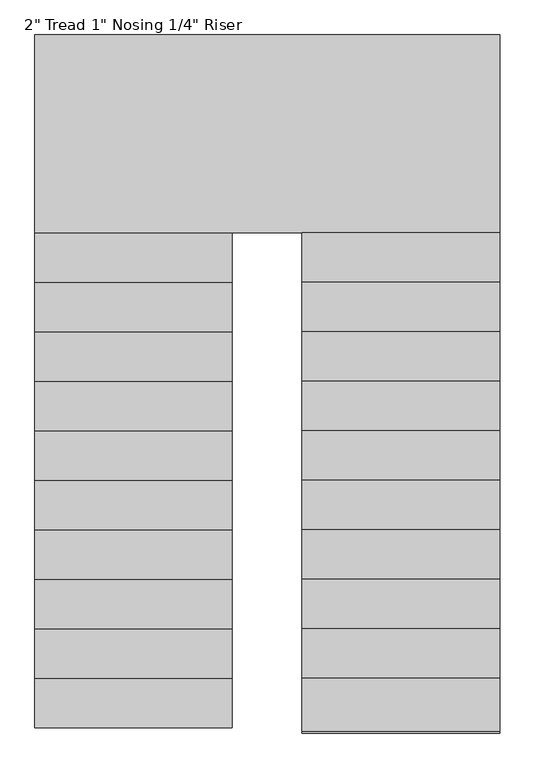
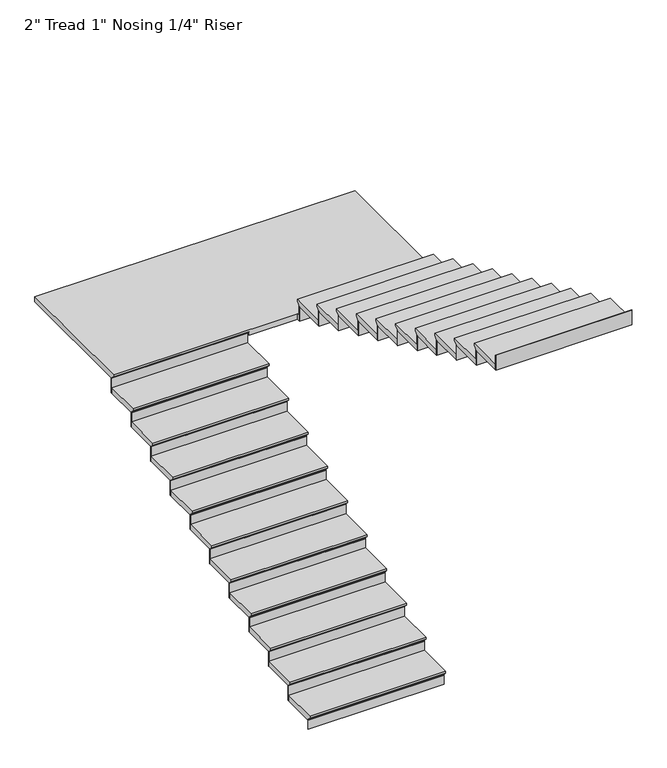
"""IFC4 building model written with IfcOpenShell, lengths in millimetres: stair flight geometry."""

from ifc_helpers import new_model, si_unit, origin, place, context, project, spatial, faceted_brep, source, transform, mapped, element, save


def stair_flight_1c36809e(model_context):
    return source(origin(), model_context, "Body", "Brep", [
        faceted_brep([(-629.5987998, 3364.6067329, 16121.4954545), (-629.5987998, 3364.6067329, 16140.5454545), (-1845.5417538, 3364.6067329, 16140.5454545), (-1845.5417538, 3364.6067329, 16121.4954545), (-629.5987998, 3390.0067329, 16096.0954545), (-1845.5417538, 3390.0067329, 16096.0954545), (-629.5987998, 3694.8067329, 16140.5454545), (-1845.5417538, 3694.8067329, 16140.5454545), (-1845.5417538, 3390.0067329, 16089.7454545), (-1845.5417538, 3694.8067329, 16089.7454545), (-629.5987998, 3694.8067329, 16089.7454545), (-629.5987998, 3390.0067329, 16089.7454545)], [[[0, 1, 2, 3]], [[4, 0, 3, 5]], [[2, 1, 6, 7]], [[8, 9, 10, 11]], [[2, 7, 9, 8, 5, 3]], [[8, 11, 4, 5]], [[6, 1, 0, 4, 11, 10]], [[7, 6, 10, 9]]]),
        faceted_brep([(-629.5987998, 3390.0067329, 16089.7454545), (-629.5987998, 3390.0067329, 16002.0), (-629.5987998, 3396.3567329, 16002.0), (-629.5987998, 3396.3567329, 16089.7454545), (-1845.5417538, 3390.0067329, 16089.7454545), (-1845.5417538, 3396.3567329, 16089.7454545), (-1845.5417538, 3396.3567329, 16002.0), (-1845.5417538, 3390.0067329, 16002.0)], [[[0, 1, 2, 3]], [[4, 5, 6, 7]], [[1, 0, 4, 7]], [[2, 1, 7, 6]], [[3, 2, 6, 5]], [[0, 3, 5, 4]]]),
        faceted_brep([(-629.5987998, 3694.8067329, 16228.2909091), (-629.5987998, 3694.8067329, 16089.7454545), (-629.5987998, 3701.1567329, 16089.7454545), (-629.5987998, 3701.1567329, 16228.2909091), (-1845.5417538, 3694.8067329, 16228.2909091), (-1845.5417538, 3701.1567329, 16228.2909091), (-1845.5417538, 3701.1567329, 16089.7454545), (-1845.5417538, 3694.8067329, 16089.7454545)], [[[0, 1, 2, 3]], [[4, 5, 6, 7]], [[1, 0, 4, 7]], [[2, 1, 7, 6]], [[3, 2, 6, 5]], [[0, 3, 5, 4]]]),
        faceted_brep([(-1845.5417538, 3669.4067329, 16279.0909091), (-629.5987998, 3669.4067329, 16279.0909091), (-629.5987998, 3999.6067329, 16279.0909091), (-1845.5417538, 3999.6067329, 16279.0909091), (-1845.5417538, 3694.8067329, 16228.2909091), (-1845.5417538, 3999.6067329, 16228.2909091), (-629.5987998, 3999.6067329, 16228.2909091), (-629.5987998, 3694.8067329, 16228.2909091), (-1845.5417538, 3694.8067329, 16234.6409091), (-1845.5417538, 3669.4067329, 16260.0409091), (-629.5987998, 3694.8067329, 16234.6409091), (-629.5987998, 3669.4067329, 16260.0409091)], [[[0, 1, 2, 3]], [[4, 5, 6, 7]], [[0, 3, 5, 4, 8, 9]], [[4, 7, 10, 8]], [[2, 1, 11, 10, 7, 6]], [[3, 2, 6, 5]], [[11, 1, 0, 9]], [[10, 11, 9, 8]]]),
        faceted_brep([(-629.5987998, 3999.6067329, 16366.8363636), (-629.5987998, 3999.6067329, 16228.2909091), (-629.5987998, 4005.9567329, 16228.2909091), (-629.5987998, 4005.9567329, 16366.8363636), (-1845.5417538, 3999.6067329, 16366.8363636), (-1845.5417538, 4005.9567329, 16366.8363636), (-1845.5417538, 4005.9567329, 16228.2909091), (-1845.5417538, 3999.6067329, 16228.2909091)], [[[0, 1, 2, 3]], [[4, 5, 6, 7]], [[1, 0, 4, 7]], [[2, 1, 7, 6]], [[3, 2, 6, 5]], [[0, 3, 5, 4]]]),
        faceted_brep([(-1845.5417538, 3974.2067329, 16417.6363636), (-629.5987998, 3974.2067329, 16417.6363636), (-629.5987998, 4304.4067329, 16417.6363636), (-1845.5417538, 4304.4067329, 16417.6363636), (-1845.5417538, 3999.6067329, 16366.8363636), (-1845.5417538, 4304.4067329, 16366.8363636), (-629.5987998, 4304.4067329, 16366.8363636), (-629.5987998, 3999.6067329, 16366.8363636), (-1845.5417538, 3999.6067329, 16373.1863636), (-1845.5417538, 3974.2067329, 16398.5863636), (-629.5987998, 3999.6067329, 16373.1863636), (-629.5987998, 3974.2067329, 16398.5863636)], [[[0, 1, 2, 3]], [[4, 5, 6, 7]], [[0, 3, 5, 4, 8, 9]], [[4, 7, 10, 8]], [[2, 1, 11, 10, 7, 6]], [[3, 2, 6, 5]], [[11, 1, 0, 9]], [[10, 11, 9, 8]]]),
        faceted_brep([(-629.5987998, 4304.4067329, 16505.3818182), (-629.5987998, 4304.4067329, 16366.8363636), (-629.5987998, 4310.7567329, 16366.8363636), (-629.5987998, 4310.7567329, 16505.3818182), (-1845.5417538, 4304.4067329, 16505.3818182), (-1845.5417538, 4310.7567329, 16505.3818182), (-1845.5417538, 4310.7567329, 16366.8363636), (-1845.5417538, 4304.4067329, 16366.8363636)], [[[0, 1, 2, 3]], [[4, 5, 6, 7]], [[1, 0, 4, 7]], [[2, 1, 7, 6]], [[3, 2, 6, 5]], [[0, 3, 5, 4]]]),
        faceted_brep([(-1845.5417538, 4279.0067329, 16556.1818182), (-629.5987998, 4279.0067329, 16556.1818182), (-629.5987998, 4609.2067329, 16556.1818182), (-1845.5417538, 4609.2067329, 16556.1818182), (-1845.5417538, 4304.4067329, 16505.3818182), (-1845.5417538, 4609.2067329, 16505.3818182), (-629.5987998, 4609.2067329, 16505.3818182), (-629.5987998, 4304.4067329, 16505.3818182), (-1845.5417538, 4304.4067329, 16511.7318182), (-1845.5417538, 4279.0067329, 16537.1318182), (-629.5987998, 4304.4067329, 16511.7318182), (-629.5987998, 4279.0067329, 16537.1318182)], [[[0, 1, 2, 3]], [[4, 5, 6, 7]], [[0, 3, 5, 4, 8, 9]], [[4, 7, 10, 8]], [[2, 1, 11, 10, 7, 6]], [[3, 2, 6, 5]], [[11, 1, 0, 9]], [[10, 11, 9, 8]]]),
        faceted_brep([(-629.5987998, 4609.2067329, 16643.9272727), (-629.5987998, 4609.2067329, 16505.3818182), (-629.5987998, 4615.5567329, 16505.3818182), (-629.5987998, 4615.5567329, 16643.9272727), (-1845.5417538, 4609.2067329, 16643.9272727), (-1845.5417538, 4615.5567329, 16643.9272727), (-1845.5417538, 4615.5567329, 16505.3818182), (-1845.5417538, 4609.2067329, 16505.3818182)], [[[0, 1, 2, 3]], [[4, 5, 6, 7]], [[1, 0, 4, 7]], [[2, 1, 7, 6]], [[3, 2, 6, 5]], [[0, 3, 5, 4]]]),
        faceted_brep([(-1845.5417538, 4583.8067329, 16694.7272727), (-629.5987998, 4583.8067329, 16694.7272727), (-629.5987998, 4914.0067329, 16694.7272727), (-1845.5417538, 4914.0067329, 16694.7272727), (-1845.5417538, 4609.2067329, 16643.9272727), (-1845.5417538, 4914.0067329, 16643.9272727), (-629.5987998, 4914.0067329, 16643.9272727), (-629.5987998, 4609.2067329, 16643.9272727), (-1845.5417538, 4609.2067329, 16650.2772727), (-1845.5417538, 4583.8067329, 16675.6772727), (-629.5987998, 4609.2067329, 16650.2772727), (-629.5987998, 4583.8067329, 16675.6772727)], [[[0, 1, 2, 3]], [[4, 5, 6, 7]], [[0, 3, 5, 4, 8, 9]], [[4, 7, 10, 8]], [[2, 1, 11, 10, 7, 6]], [[3, 2, 6, 5]], [[11, 1, 0, 9]], [[10, 11, 9, 8]]]),
        faceted_brep([(-629.5987998, 4914.0067329, 16782.4727273), (-629.5987998, 4914.0067329, 16643.9272727), (-629.5987998, 4920.3567329, 16643.9272727), (-629.5987998, 4920.3567329, 16782.4727273), (-1845.5417538, 4914.0067329, 16782.4727273), (-1845.5417538, 4920.3567329, 16782.4727273), (-1845.5417538, 4920.3567329, 16643.9272727), (-1845.5417538, 4914.0067329, 16643.9272727)], [[[0, 1, 2, 3]], [[4, 5, 6, 7]], [[1, 0, 4, 7]], [[2, 1, 7, 6]], [[3, 2, 6, 5]], [[0, 3, 5, 4]]]),
        faceted_brep([(-1845.5417538, 4888.6067329, 16833.2727273), (-629.5987998, 4888.6067329, 16833.2727273), (-629.5987998, 5218.8067329, 16833.2727273), (-1845.5417538, 5218.8067329, 16833.2727273), (-1845.5417538, 4914.0067329, 16782.4727273), (-1845.5417538, 5218.8067329, 16782.4727273), (-629.5987998, 5218.8067329, 16782.4727273), (-629.5987998, 4914.0067329, 16782.4727273), (-1845.5417538, 4914.0067329, 16788.8227273), (-1845.5417538, 4888.6067329, 16814.2227273), (-629.5987998, 4914.0067329, 16788.8227273), (-629.5987998, 4888.6067329, 16814.2227273)], [[[0, 1, 2, 3]], [[4, 5, 6, 7]], [[0, 3, 5, 4, 8, 9]], [[4, 7, 10, 8]], [[2, 1, 11, 10, 7, 6]], [[3, 2, 6, 5]], [[11, 1, 0, 9]], [[10, 11, 9, 8]]]),
        faceted_brep([(-629.5987998, 5218.8067329, 16921.0181818), (-629.5987998, 5218.8067329, 16782.4727273), (-629.5987998, 5225.1567329, 16782.4727273), (-629.5987998, 5225.1567329, 16921.0181818), (-1845.5417538, 5218.8067329, 16921.0181818), (-1845.5417538, 5225.1567329, 16921.0181818), (-1845.5417538, 5225.1567329, 16782.4727273), (-1845.5417538, 5218.8067329, 16782.4727273)], [[[0, 1, 2, 3]], [[4, 5, 6, 7]], [[1, 0, 4, 7]], [[2, 1, 7, 6]], [[3, 2, 6, 5]], [[0, 3, 5, 4]]]),
        faceted_brep([(-1845.5417538, 5193.4067329, 16971.8181818), (-629.5987998, 5193.4067329, 16971.8181818), (-629.5987998, 5523.6067329, 16971.8181818), (-1845.5417538, 5523.6067329, 16971.8181818), (-1845.5417538, 5218.8067329, 16921.0181818), (-1845.5417538, 5523.6067329, 16921.0181818), (-629.5987998, 5523.6067329, 16921.0181818), (-629.5987998, 5218.8067329, 16921.0181818), (-1845.5417538, 5218.8067329, 16927.3681818), (-1845.5417538, 5193.4067329, 16952.7681818), (-629.5987998, 5218.8067329, 16927.3681818), (-629.5987998, 5193.4067329, 16952.7681818)], [[[0, 1, 2, 3]], [[4, 5, 6, 7]], [[0, 3, 5, 4, 8, 9]], [[4, 7, 10, 8]], [[2, 1, 11, 10, 7, 6]], [[3, 2, 6, 5]], [[11, 1, 0, 9]], [[10, 11, 9, 8]]]),
        faceted_brep([(-629.5987998, 5523.6067329, 17059.5636364), (-629.5987998, 5523.6067329, 16921.0181818), (-629.5987998, 5529.9567329, 16921.0181818), (-629.5987998, 5529.9567329, 17059.5636364), (-1845.5417538, 5523.6067329, 17059.5636364), (-1845.5417538, 5529.9567329, 17059.5636364), (-1845.5417538, 5529.9567329, 16921.0181818), (-1845.5417538, 5523.6067329, 16921.0181818)], [[[0, 1, 2, 3]], [[4, 5, 6, 7]], [[1, 0, 4, 7]], [[2, 1, 7, 6]], [[3, 2, 6, 5]], [[0, 3, 5, 4]]]),
        faceted_brep([(-1845.5417538, 5498.2067329, 17110.3636364), (-629.5987998, 5498.2067329, 17110.3636364), (-629.5987998, 5828.4067329, 17110.3636364), (-1845.5417538, 5828.4067329, 17110.3636364), (-1845.5417538, 5523.6067329, 17059.5636364), (-1845.5417538, 5828.4067329, 17059.5636364), (-629.5987998, 5828.4067329, 17059.5636364), (-629.5987998, 5523.6067329, 17059.5636364), (-1845.5417538, 5523.6067329, 17065.9136364), (-1845.5417538, 5498.2067329, 17091.3136364), (-629.5987998, 5523.6067329, 17065.9136364), (-629.5987998, 5498.2067329, 17091.3136364)], [[[0, 1, 2, 3]], [[4, 5, 6, 7]], [[0, 3, 5, 4, 8, 9]], [[4, 7, 10, 8]], [[2, 1, 11, 10, 7, 6]], [[3, 2, 6, 5]], [[11, 1, 0, 9]], [[10, 11, 9, 8]]]),
        faceted_brep([(-629.5987998, 5828.4067329, 17198.1090909), (-629.5987998, 5828.4067329, 17059.5636364), (-629.5987998, 5834.7567329, 17059.5636364), (-629.5987998, 5834.7567329, 17198.1090909), (-1845.5417538, 5828.4067329, 17198.1090909), (-1845.5417538, 5834.7567329, 17198.1090909), (-1845.5417538, 5834.7567329, 17059.5636364), (-1845.5417538, 5828.4067329, 17059.5636364)], [[[0, 1, 2, 3]], [[4, 5, 6, 7]], [[1, 0, 4, 7]], [[2, 1, 7, 6]], [[3, 2, 6, 5]], [[0, 3, 5, 4]]]),
        faceted_brep([(-1845.5417538, 5803.0067329, 17248.9090909), (-629.5987998, 5803.0067329, 17248.9090909), (-629.5987998, 6133.2067329, 17248.9090909), (-1845.5417538, 6133.2067329, 17248.9090909), (-1845.5417538, 5828.4067329, 17198.1090909), (-1845.5417538, 6133.2067329, 17198.1090909), (-629.5987998, 6133.2067329, 17198.1090909), (-629.5987998, 5828.4067329, 17198.1090909), (-1845.5417538, 5828.4067329, 17204.4590909), (-1845.5417538, 5803.0067329, 17229.8590909), (-629.5987998, 5828.4067329, 17204.4590909), (-629.5987998, 5803.0067329, 17229.8590909)], [[[0, 1, 2, 3]], [[4, 5, 6, 7]], [[0, 3, 5, 4, 8, 9]], [[4, 7, 10, 8]], [[2, 1, 11, 10, 7, 6]], [[3, 2, 6, 5]], [[11, 1, 0, 9]], [[10, 11, 9, 8]]]),
        faceted_brep([(-629.5987998, 6133.2067329, 17336.6545455), (-629.5987998, 6133.2067329, 17198.1090909), (-629.5987998, 6139.5567329, 17198.1090909), (-629.5987998, 6139.5567329, 17336.6545455), (-1845.5417538, 6133.2067329, 17336.6545455), (-1845.5417538, 6139.5567329, 17336.6545455), (-1845.5417538, 6139.5567329, 17198.1090909), (-1845.5417538, 6133.2067329, 17198.1090909)], [[[0, 1, 2, 3]], [[4, 5, 6, 7]], [[1, 0, 4, 7]], [[2, 1, 7, 6]], [[3, 2, 6, 5]], [[0, 3, 5, 4]]]),
        faceted_brep([(-1845.5417538, 6107.8067329, 17387.4545455), (-629.5987998, 6107.8067329, 17387.4545455), (-629.5987998, 6438.0067329, 17387.4545455), (-1845.5417538, 6438.0067329, 17387.4545455), (-1845.5417538, 6133.2067329, 17336.6545455), (-1845.5417538, 6438.0067329, 17336.6545455), (-629.5987998, 6438.0067329, 17336.6545455), (-629.5987998, 6133.2067329, 17336.6545455), (-1845.5417538, 6133.2067329, 17343.0045455), (-1845.5417538, 6107.8067329, 17368.4045455), (-629.5987998, 6133.2067329, 17343.0045455), (-629.5987998, 6107.8067329, 17368.4045455)], [[[0, 1, 2, 3]], [[4, 5, 6, 7]], [[0, 3, 5, 4, 8, 9]], [[4, 7, 10, 8]], [[2, 1, 11, 10, 7, 6]], [[3, 2, 6, 5]], [[11, 1, 0, 9]], [[10, 11, 9, 8]]]),
        faceted_brep([(-629.5987998, 6438.0067329, 17475.2), (-629.5987998, 6438.0067329, 17336.6545455), (-629.5987998, 6444.3567329, 17336.6545455), (-629.5987998, 6444.3567329, 17475.2), (-1845.5417538, 6438.0067329, 17475.2), (-1845.5417538, 6444.3567329, 17475.2), (-1845.5417538, 6444.3567329, 17336.6545455), (-1845.5417538, 6438.0067329, 17336.6545455)], [[[0, 1, 2, 3]], [[4, 5, 6, 7]], [[1, 0, 4, 7]], [[2, 1, 7, 6]], [[3, 2, 6, 5]], [[0, 3, 5, 4]]]),
        faceted_brep([(1021.4012085, 6387.2067329, 17526.0), (1021.4012085, 7631.8067329, 17526.0), (-1845.5417538, 7631.8067329, 17526.0), (-1845.5417538, 6412.6067329, 17526.0), (-197.7987915, 6412.6067329, 17526.0), (-197.7987915, 6387.2067329, 17526.0), (1021.4012085, 7631.8067329, 17475.2), (1021.4012085, 6387.2067329, 17475.2), (-197.7987915, 6387.2067329, 17475.2), (-197.7987915, 6412.6067329, 17475.2), (-629.5987998, 6412.6067329, 17475.2), (-629.5987998, 6438.0067329, 17475.2), (-1845.5417538, 6438.0067329, 17475.2), (-1845.5417538, 7631.8067329, 17475.2), (-629.5987998, 6438.0067329, 17481.55), (-1845.5417538, 6438.0067329, 17481.55), (-1845.5417538, 6412.6067329, 17506.95), (-629.5987998, 6412.6067329, 17506.95)], [[[0, 1, 2, 3, 4, 5]], [[6, 7, 8, 9, 10, 11, 12, 13]], [[1, 0, 7, 6]], [[2, 1, 6, 13]], [[12, 11, 14, 15]], [[4, 3, 16, 17, 10, 9]], [[5, 4, 9, 8]], [[0, 5, 8, 7]], [[16, 15, 14, 17]], [[3, 2, 13, 12, 15, 16]], [[11, 10, 17, 14]]]),
        faceted_brep([(-197.7987915, 6387.2067329, 17613.7454545), (-197.7987915, 6387.2067329, 17475.2), (-197.7987915, 6380.8567329, 17475.2), (-197.7987915, 6380.8567329, 17613.7454545), (1021.4012085, 6387.2067329, 17613.7454545), (1021.4012085, 6380.8567329, 17613.7454545), (1021.4012085, 6380.8567329, 17475.2), (1021.4012085, 6387.2067329, 17475.2)], [[[0, 1, 2, 3]], [[4, 5, 6, 7]], [[1, 0, 4, 7]], [[2, 1, 7, 6]], [[3, 2, 6, 5]], [[0, 3, 5, 4]]]),
        faceted_brep([(1021.4012085, 6412.6067329, 17664.5454545), (-197.7987915, 6412.6067329, 17664.5454545), (-197.7987915, 6082.4067329, 17664.5454545), (1021.4012085, 6082.4067329, 17664.5454545), (1021.4012085, 6387.2067329, 17613.7454545), (1021.4012085, 6082.4067329, 17613.7454545), (-197.7987915, 6082.4067329, 17613.7454545), (-197.7987915, 6387.2067329, 17613.7454545), (1021.4012085, 6387.2067329, 17620.0954545), (1021.4012085, 6412.6067329, 17645.4954545), (-197.7987915, 6387.2067329, 17620.0954545), (-197.7987915, 6412.6067329, 17645.4954545)], [[[0, 1, 2, 3]], [[4, 5, 6, 7]], [[0, 3, 5, 4, 8, 9]], [[4, 7, 10, 8]], [[2, 1, 11, 10, 7, 6]], [[3, 2, 6, 5]], [[11, 1, 0, 9]], [[10, 11, 9, 8]]]),
        faceted_brep([(-197.7987915, 6082.4067329, 17752.2909091), (-197.7987915, 6082.4067329, 17613.7454545), (-197.7987915, 6076.0567329, 17613.7454545), (-197.7987915, 6076.0567329, 17752.2909091), (1021.4012085, 6082.4067329, 17752.2909091), (1021.4012085, 6076.0567329, 17752.2909091), (1021.4012085, 6076.0567329, 17613.7454545), (1021.4012085, 6082.4067329, 17613.7454545)], [[[0, 1, 2, 3]], [[4, 5, 6, 7]], [[1, 0, 4, 7]], [[2, 1, 7, 6]], [[3, 2, 6, 5]], [[0, 3, 5, 4]]]),
        faceted_brep([(1021.4012085, 6107.8067329, 17803.0909091), (-197.7987915, 6107.8067329, 17803.0909091), (-197.7987915, 5777.6067329, 17803.0909091), (1021.4012085, 5777.6067329, 17803.0909091), (1021.4012085, 6082.4067329, 17752.2909091), (1021.4012085, 5777.6067329, 17752.2909091), (-197.7987915, 5777.6067329, 17752.2909091), (-197.7987915, 6082.4067329, 17752.2909091), (1021.4012085, 6082.4067329, 17758.6409091), (1021.4012085, 6107.8067329, 17784.0409091), (-197.7987915, 6082.4067329, 17758.6409091), (-197.7987915, 6107.8067329, 17784.0409091)], [[[0, 1, 2, 3]], [[4, 5, 6, 7]], [[0, 3, 5, 4, 8, 9]], [[4, 7, 10, 8]], [[2, 1, 11, 10, 7, 6]], [[3, 2, 6, 5]], [[11, 1, 0, 9]], [[10, 11, 9, 8]]]),
        faceted_brep([(-197.7987915, 5777.6067329, 17890.8363636), (-197.7987915, 5777.6067329, 17752.2909091), (-197.7987915, 5771.2567329, 17752.2909091), (-197.7987915, 5771.2567329, 17890.8363636), (1021.4012085, 5777.6067329, 17890.8363636), (1021.4012085, 5771.2567329, 17890.8363636), (1021.4012085, 5771.2567329, 17752.2909091), (1021.4012085, 5777.6067329, 17752.2909091)], [[[0, 1, 2, 3]], [[4, 5, 6, 7]], [[1, 0, 4, 7]], [[2, 1, 7, 6]], [[3, 2, 6, 5]], [[0, 3, 5, 4]]]),
        faceted_brep([(1021.4012085, 5803.0067329, 17941.6363636), (-197.7987915, 5803.0067329, 17941.6363636), (-197.7987915, 5472.8067329, 17941.6363636), (1021.4012085, 5472.8067329, 17941.6363636), (1021.4012085, 5777.6067329, 17890.8363636), (1021.4012085, 5472.8067329, 17890.8363636), (-197.7987915, 5472.8067329, 17890.8363636), (-197.7987915, 5777.6067329, 17890.8363636), (1021.4012085, 5777.6067329, 17897.1863636), (1021.4012085, 5803.0067329, 17922.5863636), (-197.7987915, 5777.6067329, 17897.1863636), (-197.7987915, 5803.0067329, 17922.5863636)], [[[0, 1, 2, 3]], [[4, 5, 6, 7]], [[0, 3, 5, 4, 8, 9]], [[4, 7, 10, 8]], [[2, 1, 11, 10, 7, 6]], [[3, 2, 6, 5]], [[11, 1, 0, 9]], [[10, 11, 9, 8]]]),
        faceted_brep([(-197.7987915, 5472.8067329, 18029.3818182), (-197.7987915, 5472.8067329, 17890.8363636), (-197.7987915, 5466.4567329, 17890.8363636), (-197.7987915, 5466.4567329, 18029.3818182), (1021.4012085, 5472.8067329, 18029.3818182), (1021.4012085, 5466.4567329, 18029.3818182), (1021.4012085, 5466.4567329, 17890.8363636), (1021.4012085, 5472.8067329, 17890.8363636)], [[[0, 1, 2, 3]], [[4, 5, 6, 7]], [[1, 0, 4, 7]], [[2, 1, 7, 6]], [[3, 2, 6, 5]], [[0, 3, 5, 4]]]),
        faceted_brep([(1021.4012085, 5498.2067329, 18080.1818182), (-197.7987915, 5498.2067329, 18080.1818182), (-197.7987915, 5168.0067329, 18080.1818182), (1021.4012085, 5168.0067329, 18080.1818182), (1021.4012085, 5472.8067329, 18029.3818182), (1021.4012085, 5168.0067329, 18029.3818182), (-197.7987915, 5168.0067329, 18029.3818182), (-197.7987915, 5472.8067329, 18029.3818182), (1021.4012085, 5472.8067329, 18035.7318182), (1021.4012085, 5498.2067329, 18061.1318182), (-197.7987915, 5472.8067329, 18035.7318182), (-197.7987915, 5498.2067329, 18061.1318182)], [[[0, 1, 2, 3]], [[4, 5, 6, 7]], [[0, 3, 5, 4, 8, 9]], [[4, 7, 10, 8]], [[2, 1, 11, 10, 7, 6]], [[3, 2, 6, 5]], [[11, 1, 0, 9]], [[10, 11, 9, 8]]]),
        faceted_brep([(-197.7987915, 5168.0067329, 18167.9272727), (-197.7987915, 5168.0067329, 18029.3818182), (-197.7987915, 5161.6567329, 18029.3818182), (-197.7987915, 5161.6567329, 18167.9272727), (1021.4012085, 5168.0067329, 18167.9272727), (1021.4012085, 5161.6567329, 18167.9272727), (1021.4012085, 5161.6567329, 18029.3818182), (1021.4012085, 5168.0067329, 18029.3818182)], [[[0, 1, 2, 3]], [[4, 5, 6, 7]], [[1, 0, 4, 7]], [[2, 1, 7, 6]], [[3, 2, 6, 5]], [[0, 3, 5, 4]]]),
        faceted_brep([(1021.4012085, 5193.4067329, 18218.7272727), (-197.7987915, 5193.4067329, 18218.7272727), (-197.7987915, 4863.2067329, 18218.7272727), (1021.4012085, 4863.2067329, 18218.7272727), (1021.4012085, 5168.0067329, 18167.9272727), (1021.4012085, 4863.2067329, 18167.9272727), (-197.7987915, 4863.2067329, 18167.9272727), (-197.7987915, 5168.0067329, 18167.9272727), (1021.4012085, 5168.0067329, 18174.2772727), (1021.4012085, 5193.4067329, 18199.6772727), (-197.7987915, 5168.0067329, 18174.2772727), (-197.7987915, 5193.4067329, 18199.6772727)], [[[0, 1, 2, 3]], [[4, 5, 6, 7]], [[0, 3, 5, 4, 8, 9]], [[4, 7, 10, 8]], [[2, 1, 11, 10, 7, 6]], [[3, 2, 6, 5]], [[11, 1, 0, 9]], [[10, 11, 9, 8]]]),
        faceted_brep([(-197.7987915, 4863.2067329, 18306.4727273), (-197.7987915, 4863.2067329, 18167.9272727), (-197.7987915, 4856.8567329, 18167.9272727), (-197.7987915, 4856.8567329, 18306.4727273), (1021.4012085, 4863.2067329, 18306.4727273), (1021.4012085, 4856.8567329, 18306.4727273), (1021.4012085, 4856.8567329, 18167.9272727), (1021.4012085, 4863.2067329, 18167.9272727)], [[[0, 1, 2, 3]], [[4, 5, 6, 7]], [[1, 0, 4, 7]], [[2, 1, 7, 6]], [[3, 2, 6, 5]], [[0, 3, 5, 4]]]),
        faceted_brep([(1021.4012085, 4888.6067329, 18357.2727273), (-197.7987915, 4888.6067329, 18357.2727273), (-197.7987915, 4558.4067329, 18357.2727273), (1021.4012085, 4558.4067329, 18357.2727273), (1021.4012085, 4863.2067329, 18306.4727273), (1021.4012085, 4558.4067329, 18306.4727273), (-197.7987915, 4558.4067329, 18306.4727273), (-197.7987915, 4863.2067329, 18306.4727273), (1021.4012085, 4863.2067329, 18312.8227273), (1021.4012085, 4888.6067329, 18338.2227273), (-197.7987915, 4863.2067329, 18312.8227273), (-197.7987915, 4888.6067329, 18338.2227273)], [[[0, 1, 2, 3]], [[4, 5, 6, 7]], [[0, 3, 5, 4, 8, 9]], [[4, 7, 10, 8]], [[2, 1, 11, 10, 7, 6]], [[3, 2, 6, 5]], [[11, 1, 0, 9]], [[10, 11, 9, 8]]]),
        faceted_brep([(-197.7987915, 4558.4067329, 18445.0181818), (-197.7987915, 4558.4067329, 18306.4727273), (-197.7987915, 4552.0567329, 18306.4727273), (-197.7987915, 4552.0567329, 18445.0181818), (1021.4012085, 4558.4067329, 18445.0181818), (1021.4012085, 4552.0567329, 18445.0181818), (1021.4012085, 4552.0567329, 18306.4727273), (1021.4012085, 4558.4067329, 18306.4727273)], [[[0, 1, 2, 3]], [[4, 5, 6, 7]], [[1, 0, 4, 7]], [[2, 1, 7, 6]], [[3, 2, 6, 5]], [[0, 3, 5, 4]]]),
        faceted_brep([(1021.4012085, 4583.8067329, 18495.8181818), (-197.7987915, 4583.8067329, 18495.8181818), (-197.7987915, 4253.6067329, 18495.8181818), (1021.4012085, 4253.6067329, 18495.8181818), (1021.4012085, 4558.4067329, 18445.0181818), (1021.4012085, 4253.6067329, 18445.0181818), (-197.7987915, 4253.6067329, 18445.0181818), (-197.7987915, 4558.4067329, 18445.0181818), (1021.4012085, 4558.4067329, 18451.3681818), (1021.4012085, 4583.8067329, 18476.7681818), (-197.7987915, 4558.4067329, 18451.3681818), (-197.7987915, 4583.8067329, 18476.7681818)], [[[0, 1, 2, 3]], [[4, 5, 6, 7]], [[0, 3, 5, 4, 8, 9]], [[4, 7, 10, 8]], [[2, 1, 11, 10, 7, 6]], [[3, 2, 6, 5]], [[11, 1, 0, 9]], [[10, 11, 9, 8]]]),
        faceted_brep([(-197.7987915, 4253.6067329, 18583.5636364), (-197.7987915, 4253.6067329, 18445.0181818), (-197.7987915, 4247.2567329, 18445.0181818), (-197.7987915, 4247.2567329, 18583.5636364), (1021.4012085, 4253.6067329, 18583.5636364), (1021.4012085, 4247.2567329, 18583.5636364), (1021.4012085, 4247.2567329, 18445.0181818), (1021.4012085, 4253.6067329, 18445.0181818)], [[[0, 1, 2, 3]], [[4, 5, 6, 7]], [[1, 0, 4, 7]], [[2, 1, 7, 6]], [[3, 2, 6, 5]], [[0, 3, 5, 4]]]),
        faceted_brep([(1021.4012085, 4279.0067329, 18634.3636364), (-197.7987915, 4279.0067329, 18634.3636364), (-197.7987915, 3948.8067329, 18634.3636364), (1021.4012085, 3948.8067329, 18634.3636364), (1021.4012085, 4253.6067329, 18583.5636364), (1021.4012085, 3948.8067329, 18583.5636364), (-197.7987915, 3948.8067329, 18583.5636364), (-197.7987915, 4253.6067329, 18583.5636364), (1021.4012085, 4253.6067329, 18589.9136364), (1021.4012085, 4279.0067329, 18615.3136364), (-197.7987915, 4253.6067329, 18589.9136364), (-197.7987915, 4279.0067329, 18615.3136364)], [[[0, 1, 2, 3]], [[4, 5, 6, 7]], [[0, 3, 5, 4, 8, 9]], [[4, 7, 10, 8]], [[2, 1, 11, 10, 7, 6]], [[3, 2, 6, 5]], [[11, 1, 0, 9]], [[10, 11, 9, 8]]]),
        faceted_brep([(-197.7987915, 3948.8067329, 18722.1090909), (-197.7987915, 3948.8067329, 18583.5636364), (-197.7987915, 3942.4567329, 18583.5636364), (-197.7987915, 3942.4567329, 18722.1090909), (1021.4012085, 3948.8067329, 18722.1090909), (1021.4012085, 3942.4567329, 18722.1090909), (1021.4012085, 3942.4567329, 18583.5636364), (1021.4012085, 3948.8067329, 18583.5636364)], [[[0, 1, 2, 3]], [[4, 5, 6, 7]], [[1, 0, 4, 7]], [[2, 1, 7, 6]], [[3, 2, 6, 5]], [[0, 3, 5, 4]]]),
        faceted_brep([(1021.4012085, 3974.2067329, 18772.9090909), (-197.7987915, 3974.2067329, 18772.9090909), (-197.7987915, 3644.0067329, 18772.9090909), (1021.4012085, 3644.0067329, 18772.9090909), (1021.4012085, 3948.8067329, 18722.1090909), (1021.4012085, 3644.0067329, 18722.1090909), (-197.7987915, 3644.0067329, 18722.1090909), (-197.7987915, 3948.8067329, 18722.1090909), (1021.4012085, 3948.8067329, 18728.4590909), (1021.4012085, 3974.2067329, 18753.8590909), (-197.7987915, 3948.8067329, 18728.4590909), (-197.7987915, 3974.2067329, 18753.8590909)], [[[0, 1, 2, 3]], [[4, 5, 6, 7]], [[0, 3, 5, 4, 8, 9]], [[4, 7, 10, 8]], [[2, 1, 11, 10, 7, 6]], [[3, 2, 6, 5]], [[11, 1, 0, 9]], [[10, 11, 9, 8]]]),
        faceted_brep([(-197.7987915, 3644.0067329, 18860.6545455), (-197.7987915, 3644.0067329, 18722.1090909), (-197.7987915, 3637.6567329, 18722.1090909), (-197.7987915, 3637.6567329, 18860.6545455), (1021.4012085, 3644.0067329, 18860.6545455), (1021.4012085, 3637.6567329, 18860.6545455), (1021.4012085, 3637.6567329, 18722.1090909), (1021.4012085, 3644.0067329, 18722.1090909)], [[[0, 1, 2, 3]], [[4, 5, 6, 7]], [[1, 0, 4, 7]], [[2, 1, 7, 6]], [[3, 2, 6, 5]], [[0, 3, 5, 4]]]),
        faceted_brep([(-197.7987915, 3339.2067329, 18999.2), (-197.7987915, 3339.2067329, 18860.6545455), (-197.7987915, 3332.8567329, 18860.6545455), (-197.7987915, 3332.8567329, 18999.2), (1021.4012085, 3339.2067329, 18999.2), (1021.4012085, 3332.8567329, 18999.2), (1021.4012085, 3332.8567329, 18860.6545455), (1021.4012085, 3339.2067329, 18860.6545455)], [[[0, 1, 2, 3]], [[4, 5, 6, 7]], [[1, 0, 4, 7]], [[2, 1, 7, 6]], [[3, 2, 6, 5]], [[0, 3, 5, 4]]]),
        faceted_brep([(1021.4012085, 3669.4067329, 18911.4545455), (-197.7987915, 3669.4067329, 18911.4545455), (-197.7987915, 3339.2067329, 18911.4545455), (1021.4012085, 3339.2067329, 18911.4545455), (1021.4012085, 3644.0067329, 18860.6545455), (1021.4012085, 3339.2067329, 18860.6545455), (-197.7987915, 3339.2067329, 18860.6545455), (-197.7987915, 3644.0067329, 18860.6545455), (1021.4012085, 3644.0067329, 18867.0045455), (1021.4012085, 3669.4067329, 18892.4045455), (-197.7987915, 3644.0067329, 18867.0045455), (-197.7987915, 3669.4067329, 18892.4045455)], [[[0, 1, 2, 3]], [[4, 5, 6, 7]], [[0, 3, 5, 4, 8, 9]], [[4, 7, 10, 8]], [[2, 1, 11, 10, 7, 6]], [[3, 2, 6, 5]], [[11, 1, 0, 9]], [[10, 11, 9, 8]]]),
    ])


if __name__ == "__main__":
    model = new_model("IFC4")
    model_context = context("Model", 3, world=origin())
    ifc_project = project(units=[si_unit("LENGTHUNIT", "METRE", prefix="MILLI")], contexts=[model_context])
    site = spatial("IfcSite", under=ifc_project)
    building = spatial("IfcBuilding", under=site)
    placement = place(None, origin())
    stair_flight_shape = stair_flight_1c36809e(model_context)
    element("IfcStairFlight", 1, ObjectType="2\" Tread 1\" Nosing 1/4\" Riser", at=placement, inside=building, context=model_context, shape_type="MappedRepresentation", body=[
        mapped(stair_flight_shape, transform((0.0, 0.0, 0.0), x_axis=(1.0, 0.0, 0.0), y_axis=(0.0, 1.0, 0.0), z_axis=(0.0, 0.0, 1.0))),
    ])
    save(model, "model.ifc")
